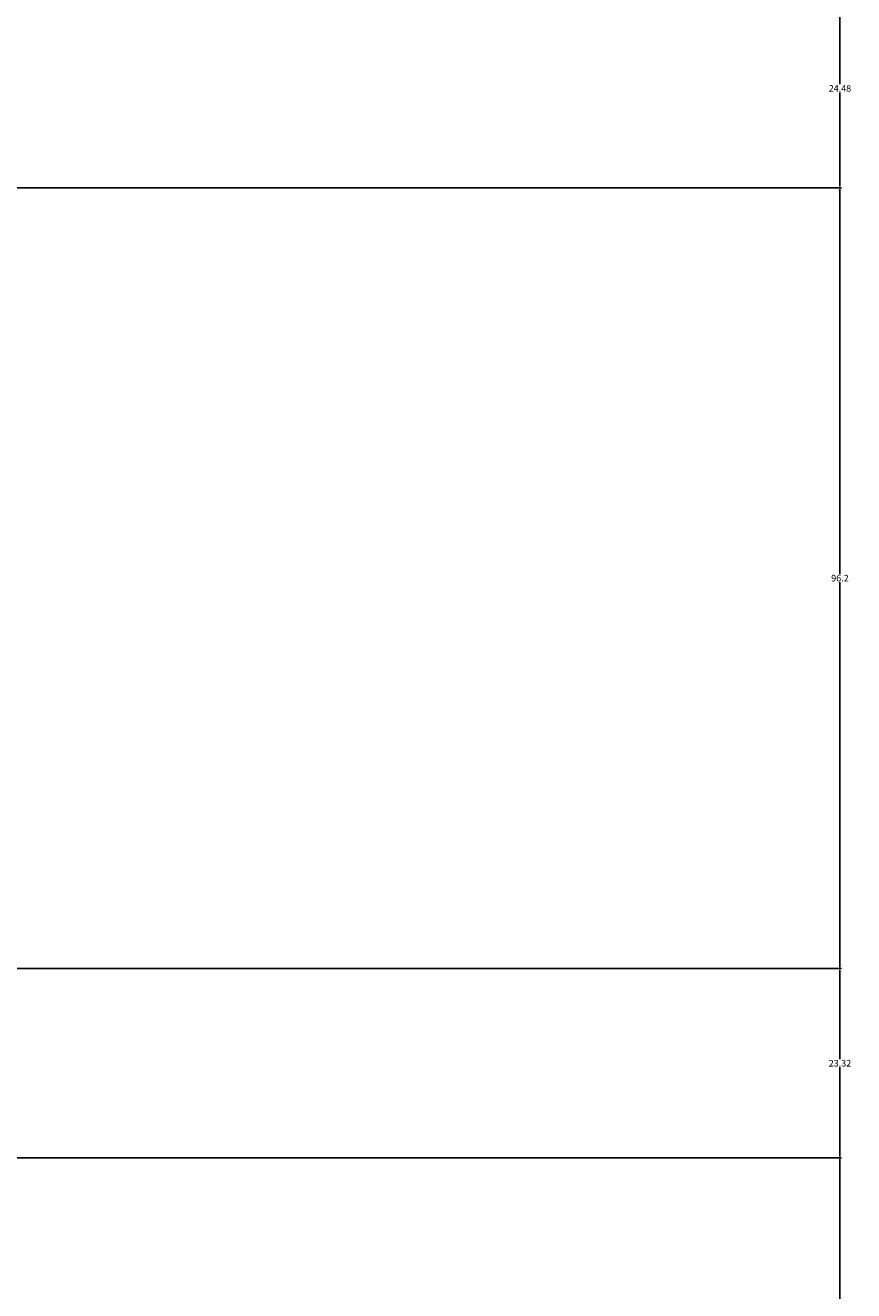
# Model space of a CAD drawing. Units: inches. Extents: x 36 to 594, y 79 to 831.
# Tile 15 of 30: x 492 to 594, y 290 to 446. Entities that reach past the tile are written whole.
import ezdxf

# ---------------------------------------------------------------- set-up
doc = ezdxf.new("R2010")
doc.units = ezdxf.units.IN
doc.header["$MEASUREMENT"] = 0
doc.layers.add('A-ANNO-DIMS', color=2, linetype='Continuous', lineweight=18)
doc.styles.get("Standard").update_dxf_attribs({"font": 'arial.ttf'})
doc.dimstyles.get("Standard").update_dxf_attribs({"dimtxt": 0.8125, "dimasz": 0.18, "dimexe": 0.18, "dimexo": 0.0625, "dimgap": 0.09, "dimtad": 0, "dimtih": 1, "dimtoh": 1, "dimdec": 4, "dimzin": 0, "dimdsep": 46, "dimlunit": 4, "dimtxsty": 'Standard', "dimcen": 0.09, "dimadec": 0, "dimazin": 0, "dimtfac": 1, "dimtdec": 4, "dimtofl": 0, "dimtmove": 0, "dimatfit": 3, "dimfxl": 1, "dimtolj": 1, "dimtzin": 0, "dimarcsym": 0})

# ---------------------------------------------------------------- blocks, each defined once
blk = doc.blocks.new('*D31')
at = {"layer": 'A-ANNO-DIMS', "color": 0, "lineweight": -2, "transparency": 16777216}
for p, q in [((448.45, 306.21), (592.85, 306.21)), ((592.67, 306.03), (592.67, 229.08)), ((592.67, 151.11), (592.67, 228.07)), ((401.61, 150.93), (592.85, 150.93))]:
    blk.add_line(p, q, dxfattribs=at)
at = {"layer": 'A-ANNO-DIMS', "color": 0, "transparency": 16777216}
for points in [[(592.64, 306.03), (592.7, 306.03), (592.67, 306.21)], [(592.64, 151.11), (592.7, 151.11), (592.67, 150.93)]]:
    blk.add_solid(points, dxfattribs=at)
at = {"layer": 'Defpoints', "color": 0, "transparency": 16777216}
for p in [(448.39, 306.21), (592.67, 306.21), (401.55, 150.93)]:
    blk.add_point(p, dxfattribs=at)
at = {"layer": 'A-ANNO-DIMS', "color": 0, "transparency": 16777216, "insert": (592.67, 228.57), "char_height": 0.812, "attachment_point": 5}
blk.add_mtext('\\A1;155.28', dxfattribs=at)
blk = doc.blocks.new('*D32')
at = {"layer": 'A-ANNO-DIMS', "color": 0, "lineweight": -2, "transparency": 16777216}
for p, q in [((424.61, 329.53), (592.85, 329.53)), ((592.67, 329.35), (592.67, 318.38)), ((592.67, 306.39), (592.67, 317.37)), ((448.45, 306.21), (592.85, 306.21))]:
    blk.add_line(p, q, dxfattribs=at)
at = {"layer": 'A-ANNO-DIMS', "color": 0, "transparency": 16777216}
for points in [[(592.64, 329.35), (592.7, 329.35), (592.67, 329.53)], [(592.64, 306.39), (592.7, 306.39), (592.67, 306.21)]]:
    blk.add_solid(points, dxfattribs=at)
at = {"layer": 'Defpoints', "color": 0, "transparency": 16777216}
for p in [(424.55, 329.53), (592.67, 329.53), (448.39, 306.21)]:
    blk.add_point(p, dxfattribs=at)
at = {"layer": 'A-ANNO-DIMS', "color": 0, "transparency": 16777216, "insert": (592.67, 317.87), "char_height": 0.812, "attachment_point": 5}
blk.add_mtext('\\A1;23.32', dxfattribs=at)
blk = doc.blocks.new('*D33')
at = {"layer": 'A-ANNO-DIMS', "color": 0, "lineweight": -2, "transparency": 16777216}
for p, q in [((424.61, 425.73), (592.85, 425.73)), ((592.67, 425.55), (592.67, 378.14)), ((592.67, 329.71), (592.67, 377.13)), ((424.61, 329.53), (592.85, 329.53))]:
    blk.add_line(p, q, dxfattribs=at)
at = {"layer": 'A-ANNO-DIMS', "color": 0, "transparency": 16777216}
for points in [[(592.64, 425.55), (592.7, 425.55), (592.67, 425.73)], [(592.64, 329.71), (592.7, 329.71), (592.67, 329.53)]]:
    blk.add_solid(points, dxfattribs=at)
at = {"layer": 'Defpoints', "color": 0, "transparency": 16777216}
for p in [(424.55, 425.73), (592.67, 425.73), (424.55, 329.53)]:
    blk.add_point(p, dxfattribs=at)
at = {"layer": 'A-ANNO-DIMS', "color": 0, "transparency": 16777216, "insert": (592.67, 377.63), "char_height": 0.812, "attachment_point": 5}
blk.add_mtext('\\A1;96.2', dxfattribs=at)
blk = doc.blocks.new('*D34')
at = {"layer": 'A-ANNO-DIMS', "color": 0, "lineweight": -2, "transparency": 16777216}
for p, q in [((448.45, 450.21), (592.85, 450.21)), ((592.67, 450.03), (592.67, 438.48)), ((592.67, 425.91), (592.67, 437.47)), ((424.61, 425.73), (592.85, 425.73))]:
    blk.add_line(p, q, dxfattribs=at)
at = {"layer": 'A-ANNO-DIMS', "color": 0, "transparency": 16777216}
for points in [[(592.64, 450.03), (592.7, 450.03), (592.67, 450.21)], [(592.64, 425.91), (592.7, 425.91), (592.67, 425.73)]]:
    blk.add_solid(points, dxfattribs=at)
at = {"layer": 'Defpoints', "color": 0, "transparency": 16777216}
for p in [(448.39, 450.21), (592.67, 450.21), (424.55, 425.73)]:
    blk.add_point(p, dxfattribs=at)
at = {"layer": 'A-ANNO-DIMS', "color": 0, "transparency": 16777216, "insert": (592.67, 437.97), "char_height": 0.812, "attachment_point": 5}
blk.add_mtext('\\A1;24.48', dxfattribs=at)

msp = doc.modelspace()

# ---------------------------------------------------------------- dimensions: what is measured, and where the dimension line sits
at = {"layer": 'A-ANNO-DIMS'}
for base, p1, p2, override, picture, middle in [((592.6689, 450.2124), (424.5492, 425.7333), (448.3898, 450.2124), {"dimdec": 2, "dimlfac": 1, "dimrnd": 0, "dimzin": 0, "dimdsep": 46, "dimlunit": 2}, '*D34', (592.6689, 437.9728)), ((592.6689, 425.7333), (424.5492, 329.5325), (424.5492, 425.7333), {"dimdec": 1, "dimlfac": 1, "dimrnd": 0, "dimzin": 0, "dimdsep": 46, "dimlunit": 2}, '*D33', (592.6689, 377.6329)), ((592.6689, 329.5325), (448.3898, 306.2124), (424.5492, 329.5325), {"dimdec": 2, "dimlfac": 1, "dimrnd": 0, "dimzin": 0, "dimdsep": 46, "dimlunit": 2}, '*D32', (592.6689, 317.8724)), ((592.6689, 306.2124), (401.5491, 150.9347), (448.3898, 306.2124), {"dimdec": 2, "dimlfac": 1, "dimrnd": 0, "dimzin": 0, "dimdsep": 46, "dimlunit": 2}, '*D31', (592.6689, 228.5735))]:
    dim = msp.add_linear_dim(base=base, p1=p1, p2=p2, angle=90, dimstyle='Standard', override=override, dxfattribs=at)
    dim.commit()
    dim.dimension.update_dxf_attribs({"geometry": picture, "text_midpoint": middle})

doc.saveas('drawing.dxf')
